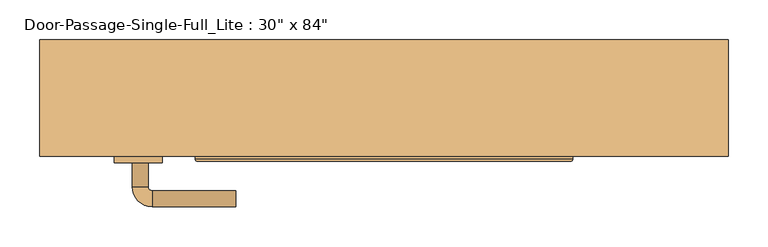
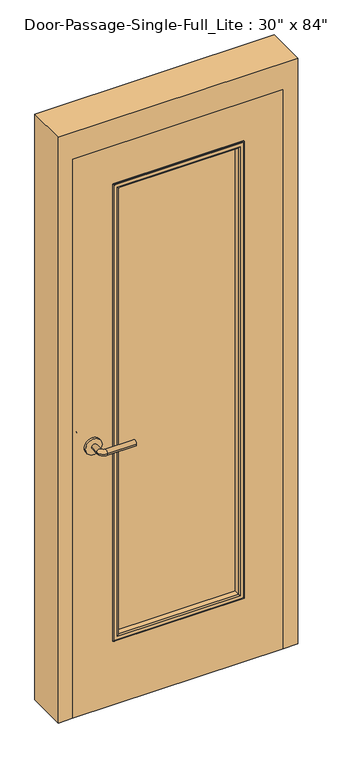
"""IFC4 building model written with IfcOpenShell, lengths in millimetres: door geometry."""

from ifc_helpers import new_model, si_unit, point, frame, frame_2d, origin, place, context, project, spatial, polyline, circle_curve, ellipse_curve, trimmed, segment, composite_curve, outline, extrude, faceted_brep, source, transform, mapped, element, save
from ifc_brep_helpers import plane_surface, cylinder_surface, revolved_surface, advanced_brep


def door_5d83ff76(model_context):
    return source(origin(), model_context, "Body", "SolidModel", [
        advanced_brep(
        [(-315.990625, -4.7, 1016.0), (-295.990625, -4.7, 1016.0), (-315.990625, 25.3, 1016.0), (-295.990625, 25.3, 1016.0), (-290.990625, 30.3, 1016.0), (-290.990625, 50.3, 1016.0), (-185.990625, 50.3, 1016.0), (-185.990625, 30.3, 1016.0)],
        [
            (0, 1, circle_curve(frame((-305.990625, -4.7, 1016.0), z_axis=(0.0, -1.0, 0.0), x_axis=(1.0, 0.0, 0.0)), 10.0)),
            (1, 0, circle_curve(frame((-305.990625, -4.7, 1016.0), z_axis=(0.0, -1.0, 0.0), x_axis=(1.0, 0.0, 0.0)), 10.0)),
            (0, 2),
            (2, 3, circle_curve(frame((-305.990625, 25.3, 1016.0), z_axis=(0.0, -1.0, 0.0), x_axis=(1.0, 0.0, 0.0)), 10.0)),
            (3, 1),
            (3, 2, circle_curve(frame((-305.990625, 25.3, 1016.0), z_axis=(0.0, -1.0, 0.0), x_axis=(1.0, 0.0, 0.0)), 10.0)),
            (4, 3, circle_curve(frame((-290.990625, 25.3, 1016.0), z_axis=(0.0, 0.0, 1.0), x_axis=(-1.0, 0.0, 0.0)), 5.0)),
            (2, 5, circle_curve(frame((-290.990625, 25.3, 1016.0), z_axis=(0.0, 0.0, -1.0), x_axis=(-1.0, 0.0, 0.0)), 25.0)),
            (5, 4, circle_curve(frame((-290.990625, 40.3, 1016.0), z_axis=(-1.0, 0.0, 0.0), x_axis=(0.0, -1.0, 0.0)), 10.0)),
            (4, 5, circle_curve(frame((-290.990625, 40.3, 1016.0), z_axis=(-1.0, 0.0, 0.0), x_axis=(0.0, -1.0, 0.0)), 10.0)),
            (6, 7, circle_curve(frame((-185.990625, 40.3, 1016.0), z_axis=(1.0, 0.0, 0.0), x_axis=(0.0, -1.0, 0.0)), 10.0)),
            (7, 6, circle_curve(frame((-185.990625, 40.3, 1016.0), z_axis=(1.0, 0.0, 0.0), x_axis=(0.0, -1.0, 0.0)), 10.0)),
            (5, 6),
            (7, 4),
        ],
        [
            plane_surface(frame((-305.990625, -4.7, 1016.0), z_axis=(0.0, -1.0, 0.0), x_axis=(0.0, 0.0, 1.0))),
            cylinder_surface(frame((-305.990625, -4.7, 1016.0), z_axis=(0.0, -1.0, 0.0), x_axis=(1.0, 0.0, 0.0)), 10.0),
            revolved_surface(trimmed(ellipse_curve(frame((-305.990625, 25.3, 1016.0), z_axis=(0.0, -1.0, 0.0), x_axis=(1.0, 0.0, 0.0)), 10.0, 10.0), [point((-315.990625, 25.3, 1016.0))], [point((-295.990625, 25.3, 1016.0))], True, "CARTESIAN"), (-290.990625, 25.3, 1016.0), (0.0, 0.0, -1.0)),
            revolved_surface(trimmed(ellipse_curve(frame((-305.990625, 25.3, 1016.0), z_axis=(0.0, -1.0, 0.0), x_axis=(1.0, 0.0, 0.0)), 10.0, 10.0), [point((-295.990625, 25.3, 1016.0))], [point((-315.990625, 25.3, 1016.0))], True, "CARTESIAN"), (-290.990625, 25.3, 1016.0), (0.0, 0.0, -1.0)),
            plane_surface(frame((-185.990625, 40.3, 1016.0), z_axis=(1.0, 0.0, 0.0), x_axis=(0.0, 0.0, 1.0))),
            cylinder_surface(frame((-290.990625, 40.3, 1016.0), z_axis=(-1.0, 0.0, 0.0), x_axis=(0.0, -1.0, 0.0)), 10.0),
        ],
        [
            (0, [[1, 2]]),
            (1, [[-1, 3, 4, 5]]),
            (1, [[-2, -5, 6, -3]]),
            (2, [[7, -4, 8, 9]]),
            (3, [[-8, -6, -7, 10]]),
            (4, [[11, 12]]),
            (5, [[-9, 13, -12, 14]]),
            (5, [[-10, -14, -11, -13]]),
        ],
    ),
        extrude(outline(composite_curve([segment(trimmed(circle_curve(frame_2d((1016.0, -308.490625)), 30.0), [point((1016.0, -338.490625))], [point((1016.0, -278.490625))], False, "CARTESIAN"), True, "CONTINUOUS"), segment(trimmed(circle_curve(frame_2d((1016.0, -308.490625)), 30.0), [point((1016.0, -278.490625))], [point((1016.0, -338.490625))], False, "CARTESIAN"), True, "CONTINUOUS")], self_intersect=False)), frame((0.0, -12.7, 0.0), z_axis=(0.0, 1.0, 0.0), x_axis=(0.0, 0.0, 1.0)), (0.0, 0.0, 1.0), 8.0),
        advanced_brep(
        [(-315.990625, -65.15, 1016.0), (-295.990625, -65.15, 1016.0), (-295.990625, -95.15, 1016.0), (-315.990625, -95.15, 1016.0), (-290.990625, -100.15, 1016.0), (-290.990625, -120.15, 1016.0), (-185.990625, -120.15, 1016.0), (-185.990625, -100.15, 1016.0)],
        [
            (0, 1, circle_curve(frame((-305.990625, -65.15, 1016.0), z_axis=(0.0, 1.0, 0.0), x_axis=(1.0, 0.0, 0.0)), 10.0)),
            (1, 0, circle_curve(frame((-305.990625, -65.15, 1016.0), z_axis=(0.0, 1.0, 0.0), x_axis=(1.0, 0.0, 0.0)), 10.0)),
            (1, 2),
            (2, 3, circle_curve(frame((-305.990625, -95.15, 1016.0), z_axis=(0.0, 1.0, 0.0), x_axis=(1.0, 0.0, 0.0)), 10.0)),
            (3, 0),
            (3, 2, circle_curve(frame((-305.990625, -95.15, 1016.0), z_axis=(0.0, 1.0, 0.0), x_axis=(1.0, 0.0, 0.0)), 10.0)),
            (4, 5, circle_curve(frame((-290.990625, -110.15, 1016.0), z_axis=(-1.0, 0.0, 0.0), x_axis=(0.0, 1.0, 0.0)), 10.0)),
            (5, 3, circle_curve(frame((-290.990625, -95.15, 1016.0), z_axis=(0.0, 0.0, -1.0), x_axis=(-1.0, 0.0, 0.0)), 25.0)),
            (2, 4, circle_curve(frame((-290.990625, -95.15, 1016.0), z_axis=(0.0, 0.0, 1.0), x_axis=(-1.0, 0.0, 0.0)), 5.0)),
            (5, 4, circle_curve(frame((-290.990625, -110.15, 1016.0), z_axis=(-1.0, 0.0, 0.0), x_axis=(0.0, 1.0, 0.0)), 10.0)),
            (6, 7, circle_curve(frame((-185.990625, -110.15, 1016.0), z_axis=(1.0, 0.0, 0.0), x_axis=(0.0, 1.0, 0.0)), 10.0)),
            (7, 6, circle_curve(frame((-185.990625, -110.15, 1016.0), z_axis=(1.0, 0.0, 0.0), x_axis=(0.0, 1.0, 0.0)), 10.0)),
            (4, 7),
            (6, 5),
        ],
        [
            plane_surface(frame((-305.990625, -65.15, 1016.0), z_axis=(0.0, 1.0, 0.0), x_axis=(0.0, 0.0, 1.0))),
            cylinder_surface(frame((-305.990625, -65.15, 1016.0), z_axis=(0.0, 1.0, 0.0), x_axis=(1.0, 0.0, 0.0)), 10.0),
            revolved_surface(trimmed(ellipse_curve(frame((-305.990625, -95.15, 1016.0), z_axis=(0.0, -1.0, 0.0), x_axis=(1.0, 0.0, 0.0)), 10.0, 10.0), [point((-315.990625, -95.15, 1016.0))], [point((-295.990625, -95.15, 1016.0))], True, "CARTESIAN"), (-290.990625, -95.15, 1016.0), (0.0, 0.0, -1.0)),
            revolved_surface(trimmed(ellipse_curve(frame((-305.990625, -95.15, 1016.0), z_axis=(0.0, -1.0, 0.0), x_axis=(1.0, 0.0, 0.0)), 10.0, 10.0), [point((-295.990625, -95.15, 1016.0))], [point((-315.990625, -95.15, 1016.0))], True, "CARTESIAN"), (-290.990625, -95.15, 1016.0), (0.0, 0.0, -1.0)),
            plane_surface(frame((-185.990625, -110.15, 1016.0), z_axis=(1.0, 0.0, 0.0), x_axis=(0.0, 0.0, 1.0))),
            cylinder_surface(frame((-290.990625, -110.15, 1016.0), z_axis=(-1.0, 0.0, 0.0), x_axis=(0.0, 1.0, 0.0)), 10.0),
        ],
        [
            (0, [[1, 2]]),
            (1, [[3, 4, 5, -2]]),
            (1, [[-5, 6, -3, -1]]),
            (2, [[7, 8, -4, 9]]),
            (3, [[10, -9, -6, -8]]),
            (4, [[11, 12]]),
            (5, [[13, -11, 14, -7]]),
            (5, [[-14, -12, -13, -10]]),
        ],
    ),
        extrude(outline(composite_curve([segment(trimmed(circle_curve(frame_2d((1016.0, -308.490625)), 30.0), [point((1016.0, -338.490625))], [point((1016.0, -278.490625))], False, "CARTESIAN"), True, "CONTINUOUS"), segment(trimmed(circle_curve(frame_2d((1016.0, -308.490625)), 30.0), [point((1016.0, -278.490625))], [point((1016.0, -338.490625))], False, "CARTESIAN"), True, "CONTINUOUS")], self_intersect=False)), frame((0.0, -65.15, 0.0), z_axis=(0.0, 1.0, 0.0), x_axis=(0.0, 0.0, 1.0)), (0.0, 0.0, 1.0), 8.0),
        extrude(outline(polyline([(228.6, -31.75), (228.6, -38.1), (-228.6, -38.1), (-228.6, -31.75), (228.6, -31.75)])), frame((0.0, 0.0, 254.0), z_axis=(0.0, 0.0, 1.0), x_axis=(1.0, 0.0, 0.0)), (0.0, 0.0, 1.0), 1727.2),
        faceted_brep([(381.0, -7.9375, 0.0), (365.125, -7.9375, 0.0), (365.125, 39.6875, 0.0), (381.0, 39.6875, 0.0), (381.0, 88.9, 0.0), (431.8, 88.9, 0.0), (431.8, -57.15, 0.0), (381.0, -57.15, 0.0), (381.0, -57.15, 2133.6), (381.0, -7.9375, 2133.6), (431.8, -57.15, 2235.2), (-431.8, -57.15, 2235.2), (-431.8, -57.15, 0.0), (-381.0, -57.15, 0.0), (-381.0, -57.15, 2133.6), (431.8, 88.9, 2235.2), (381.0, 88.9, 2133.6), (-381.0, 88.9, 2133.6), (-381.0, 88.9, 0.0), (-431.8, 88.9, 0.0), (-431.8, 88.9, 2235.2), (381.0, 39.6875, 2133.6), (365.125, 39.6875, 2117.725), (-365.125, 39.6875, 2117.725), (-365.125, 39.6875, 0.0), (-381.0, 39.6875, 0.0), (-381.0, 39.6875, 2133.6), (365.125, -7.9375, 2117.725), (-381.0, -7.9375, 2133.6), (-381.0, -7.9375, 0.0), (-365.125, -7.9375, 0.0), (-365.125, -7.9375, 2117.725)], [[[0, 1, 2, 3, 4, 5, 6, 7]], [[7, 8, 9, 0]], [[6, 10, 11, 12, 13, 14, 8, 7]], [[5, 15, 10, 6]], [[4, 16, 17, 18, 19, 20, 15, 5]], [[3, 21, 16, 4]], [[2, 22, 23, 24, 25, 26, 21, 3]], [[1, 27, 22, 2]], [[0, 9, 28, 29, 30, 31, 27, 1]], [[8, 14, 28, 9]], [[16, 21, 26, 17]], [[22, 27, 31, 23]], [[12, 19, 18, 25, 24, 30, 29, 13]], [[13, 29, 28, 14]], [[11, 20, 19, 12]], [[17, 26, 25, 18]], [[23, 31, 30, 24]], [[15, 20, 11, 10]]]),
        extrude(outline(polyline([(2133.6, -381.0), (0.0, -381.0), (0.0, 381.0), (2133.6, 381.0), (2133.6, -381.0)]), holes=[polyline([(1981.2, -228.6), (1981.2, 228.6), (254.0, 228.6), (254.0, -228.6), (1981.2, -228.6)])]), frame((0.0, -57.15, 0.0), z_axis=(0.0, 1.0, 0.0), x_axis=(0.0, 0.0, 1.0)), (0.0, 0.0, 1.0), 44.45),
        advanced_brep(
        [(-228.6, -38.1, 1981.2), (-228.6, -38.1, 254.0), (-228.6, -57.15, 254.0), (-228.6, -57.15, 1981.2), (-216.6, -58.15, 1969.2), (-216.6, -58.15, 266.0), (-216.6, -38.1, 266.0), (-216.6, -38.1, 1969.2), (-221.6, -63.15, 1974.2), (-221.6, -63.15, 261.0), (-236.6, -61.15, 1989.2), (-236.6, -61.15, 246.0), (-234.6, -63.15, 248.0), (-234.6, -63.15, 1987.2), (-236.6, -57.15, 1989.2), (-236.6, -57.15, 246.0), (228.6, -38.1, 254.0), (228.6, -57.15, 254.0), (216.6, -58.15, 266.0), (216.6, -38.1, 266.0), (221.6, -63.15, 261.0), (236.6, -61.15, 246.0), (234.6, -63.15, 248.0), (236.6, -57.15, 246.0), (228.6, -38.1, 1981.2), (228.6, -57.15, 1981.2), (216.6, -58.15, 1969.2), (216.6, -38.1, 1969.2), (221.6, -63.15, 1974.2), (236.6, -61.15, 1989.2), (234.6, -63.15, 1987.2), (236.6, -57.15, 1989.2)],
        [
            (0, 1),
            (1, 2),
            (2, 3),
            (3, 0),
            (4, 5),
            (5, 6),
            (6, 7),
            (7, 4),
            (8, 9),
            (9, 5, ellipse_curve(frame((-221.6, -58.15, 261.0), z_axis=(-0.7071067811865475, 0.0, 0.7071067811865475), x_axis=(0.7071067811865474, 0.0, 0.7071067811865476)), 7.0710678, 5.0)),
            (4, 8, ellipse_curve(frame((-221.6, -58.15, 1974.2), z_axis=(-0.7071067811865475, 0.0, -0.7071067811865475), x_axis=(-0.7071067811865474, 0.0, 0.7071067811865476)), 7.0710678, 5.0)),
            (10, 11),
            (11, 12, ellipse_curve(frame((-234.6, -61.15, 248.0), z_axis=(-0.7071067811865475, 0.0, 0.7071067811865475), x_axis=(0.7071067811865474, 0.0, 0.7071067811865476)), 2.8284271, 2.0)),
            (12, 13),
            (13, 10, ellipse_curve(frame((-234.6, -61.15, 1987.2), z_axis=(-0.7071067811865475, 0.0, -0.7071067811865475), x_axis=(-0.7071067811865474, 0.0, 0.7071067811865476)), 2.8284271, 2.0)),
            (14, 15),
            (15, 11),
            (10, 14),
            (1, 16),
            (16, 17),
            (17, 2),
            (5, 18),
            (18, 19),
            (19, 6),
            (9, 20),
            (20, 18, ellipse_curve(frame((221.6, -58.15, 261.0), z_axis=(-0.7071067811865475, 0.0, -0.7071067811865475), x_axis=(-0.7071067811865476, 0.0, 0.7071067811865474)), 7.0710678, 5.0)),
            (11, 21),
            (21, 22, ellipse_curve(frame((234.6, -61.15, 248.0), z_axis=(-0.7071067811865475, 0.0, -0.7071067811865475), x_axis=(-0.7071067811865476, 0.0, 0.7071067811865474)), 2.8284271, 2.0)),
            (22, 12),
            (15, 23),
            (23, 21),
            (16, 24),
            (24, 25),
            (25, 17),
            (18, 26),
            (26, 27),
            (27, 19),
            (20, 28),
            (28, 26, ellipse_curve(frame((221.6, -58.15, 1974.2), z_axis=(0.7071067811865475, 0.0, -0.7071067811865475), x_axis=(-0.7071067811865474, 0.0, -0.7071067811865476)), 7.0710678, 5.0)),
            (21, 29),
            (29, 30, ellipse_curve(frame((234.6, -61.15, 1987.2), z_axis=(0.7071067811865475, 0.0, -0.7071067811865475), x_axis=(-0.7071067811865474, 0.0, -0.7071067811865476)), 2.8284271, 2.0)),
            (30, 22),
            (23, 31),
            (31, 29),
            (14, 31),
            (25, 3),
            (24, 0),
            (27, 7),
            (26, 4),
            (28, 8),
            (30, 13),
            (29, 10),
        ],
        [
            plane_surface(frame((-228.6, -57.15, 1981.2), z_axis=(-1.0, 0.0, 0.0), x_axis=(0.0, 0.0, -1.0))),
            plane_surface(frame((-216.6, -38.1, 1969.2), z_axis=(1.0, 0.0, 0.0), x_axis=(0.0, 0.0, -1.0))),
            cylinder_surface(frame((-221.6, -58.15, 1981.2), z_axis=(0.0, 0.0, 1.0), x_axis=(-1.0, 0.0, 0.0)), 5.0),
            cylinder_surface(frame((-234.6, -61.15, 1981.2), z_axis=(0.0, 0.0, 1.0), x_axis=(-1.0, 0.0, 0.0)), 2.0),
            plane_surface(frame((-236.6, -61.15, 1989.2), z_axis=(-1.0, 0.0, 0.0), x_axis=(0.0, 0.0, -1.0))),
            plane_surface(frame((-228.6, -57.15, 254.0), z_axis=(0.0, 0.0, -1.0), x_axis=(1.0, 0.0, 0.0))),
            plane_surface(frame((-216.6, -38.1, 266.0), z_axis=(0.0, 0.0, 1.0), x_axis=(1.0, 0.0, 0.0))),
            cylinder_surface(frame((-228.6, -58.15, 261.0), z_axis=(-1.0, 0.0, 0.0), x_axis=(0.0, 0.0, -1.0)), 5.0),
            cylinder_surface(frame((-228.6, -61.15, 248.0), z_axis=(-1.0, 0.0, 0.0), x_axis=(0.0, 0.0, -1.0)), 2.0),
            plane_surface(frame((-236.6, -61.15, 246.0), z_axis=(0.0, 0.0, -1.0), x_axis=(1.0, 0.0, 0.0))),
            plane_surface(frame((228.6, -57.15, 254.0), z_axis=(1.0, 0.0, 0.0), x_axis=(0.0, 0.0, 1.0))),
            plane_surface(frame((216.6, -38.1, 266.0), z_axis=(-1.0, 0.0, 0.0), x_axis=(0.0, 0.0, 1.0))),
            cylinder_surface(frame((221.6, -58.15, 254.0), z_axis=(0.0, 0.0, -1.0), x_axis=(1.0, 0.0, 0.0)), 5.0),
            cylinder_surface(frame((234.6, -61.15, 254.0), z_axis=(0.0, 0.0, -1.0), x_axis=(1.0, 0.0, 0.0)), 2.0),
            plane_surface(frame((236.6, -61.15, 246.0), z_axis=(1.0, 0.0, 0.0), x_axis=(0.0, 0.0, 1.0))),
            plane_surface(frame((236.6, -57.15, 1989.2), z_axis=(0.0, 1.0, 0.0), x_axis=(-1.0, 0.0, 0.0))),
            plane_surface(frame((228.6, -57.15, 1981.2), z_axis=(0.0, 0.0, 1.0), x_axis=(-1.0, 0.0, 0.0))),
            plane_surface(frame((228.6, -38.1, 1981.2), z_axis=(0.0, 1.0, 0.0), x_axis=(-1.0, 0.0, 0.0))),
            plane_surface(frame((216.6, -38.1, 1969.2), z_axis=(0.0, 0.0, -1.0), x_axis=(-1.0, 0.0, 0.0))),
            cylinder_surface(frame((228.6, -58.15, 1974.2), z_axis=(1.0, 0.0, 0.0), x_axis=(0.0, 0.0, 1.0)), 5.0),
            plane_surface(frame((221.6, -63.15, 1974.2), z_axis=(0.0, -1.0, 0.0), x_axis=(-1.0, 0.0, 0.0))),
            cylinder_surface(frame((228.6, -61.15, 1987.2), z_axis=(1.0, 0.0, 0.0), x_axis=(0.0, 0.0, 1.0)), 2.0),
            plane_surface(frame((236.6, -61.15, 1989.2), z_axis=(0.0, 0.0, 1.0), x_axis=(-1.0, 0.0, 0.0))),
        ],
        [
            (0, [[1, 2, 3, 4]]),
            (1, [[5, 6, 7, 8]]),
            (2, [[9, 10, -5, 11]]),
            (3, [[12, 13, 14, 15]]),
            (4, [[16, 17, -12, 18]]),
            (5, [[19, 20, 21, -2]]),
            (6, [[22, 23, 24, -6]]),
            (7, [[25, 26, -22, -10]]),
            (8, [[27, 28, 29, -13]]),
            (9, [[30, 31, -27, -17]]),
            (10, [[32, 33, 34, -20]]),
            (11, [[35, 36, 37, -23]]),
            (12, [[38, 39, -35, -26]]),
            (13, [[40, 41, 42, -28]]),
            (14, [[43, 44, -40, -31]]),
            (15, [[-16, 45, -43, -30], [-3, -21, -34, 46]]),
            (16, [[47, -4, -46, -33]]),
            (17, [[-1, -47, -32, -19], [-7, -24, -37, 48]]),
            (18, [[49, -8, -48, -36]]),
            (19, [[50, -11, -49, -39]]),
            (20, [[-14, -29, -42, 51], [-9, -50, -38, -25]]),
            (21, [[52, -15, -51, -41]]),
            (22, [[-45, -18, -52, -44]]),
        ],
    ),
        advanced_brep(
        [(-228.6, -31.75, 254.0), (-228.6, -31.75, 1981.2), (-228.6, -12.7, 1981.2), (-228.6, -12.7, 254.0), (-216.6, -11.7, 266.0), (-216.6, -11.7, 1969.2), (-216.6, -31.75, 1969.2), (-216.6, -31.75, 266.0), (-221.6, -6.7, 261.0), (-221.6, -6.7, 1974.2), (-236.6, -8.7, 246.0), (-236.6, -8.7, 1989.2), (-234.6, -6.7, 1987.2), (-234.6, -6.7, 248.0), (-236.6, -12.7, 246.0), (-236.6, -12.7, 1989.2), (228.6, -31.75, 1981.2), (228.6, -12.7, 1981.2), (216.6, -11.7, 1969.2), (216.6, -31.75, 1969.2), (221.6, -6.7, 1974.2), (236.6, -8.7, 1989.2), (234.6, -6.7, 1987.2), (236.6, -12.7, 1989.2), (228.6, -31.75, 254.0), (228.6, -12.7, 254.0), (216.6, -11.7, 266.0), (216.6, -31.75, 266.0), (221.6, -6.7, 261.0), (236.6, -8.7, 246.0), (234.6, -6.7, 248.0), (236.6, -12.7, 246.0)],
        [
            (0, 1),
            (1, 2),
            (2, 3),
            (3, 0),
            (4, 5),
            (5, 6),
            (6, 7),
            (7, 4),
            (8, 9),
            (9, 5, ellipse_curve(frame((-221.6, -11.7, 1974.2), z_axis=(-0.7071067811865475, 0.0, -0.7071067811865475), x_axis=(0.7071067811865474, 0.0, -0.7071067811865476)), 7.0710678, 5.0)),
            (4, 8, ellipse_curve(frame((-221.6, -11.7, 261.0), z_axis=(-0.7071067811865475, 0.0, 0.7071067811865475), x_axis=(-0.7071067811865474, 0.0, -0.7071067811865476)), 7.0710678, 5.0)),
            (10, 11),
            (11, 12, ellipse_curve(frame((-234.6, -8.7, 1987.2), z_axis=(-0.7071067811865475, 0.0, -0.7071067811865475), x_axis=(0.7071067811865474, 0.0, -0.7071067811865476)), 2.8284271, 2.0)),
            (12, 13),
            (13, 10, ellipse_curve(frame((-234.6, -8.7, 248.0), z_axis=(-0.7071067811865475, 0.0, 0.7071067811865475), x_axis=(-0.7071067811865474, 0.0, -0.7071067811865476)), 2.8284271, 2.0)),
            (14, 15),
            (15, 11),
            (10, 14),
            (1, 16),
            (16, 17),
            (17, 2),
            (5, 18),
            (18, 19),
            (19, 6),
            (9, 20),
            (20, 18, ellipse_curve(frame((221.6, -11.7, 1974.2), z_axis=(-0.7071067811865475, 0.0, 0.7071067811865475), x_axis=(-0.7071067811865476, 0.0, -0.7071067811865474)), 7.0710678, 5.0)),
            (11, 21),
            (21, 22, ellipse_curve(frame((234.6, -8.7, 1987.2), z_axis=(-0.7071067811865475, 0.0, 0.7071067811865475), x_axis=(-0.7071067811865476, 0.0, -0.7071067811865474)), 2.8284271, 2.0)),
            (22, 12),
            (15, 23),
            (23, 21),
            (16, 24),
            (24, 25),
            (25, 17),
            (18, 26),
            (26, 27),
            (27, 19),
            (20, 28),
            (28, 26, ellipse_curve(frame((221.6, -11.7, 261.0), z_axis=(0.7071067811865475, 0.0, 0.7071067811865475), x_axis=(-0.7071067811865474, 0.0, 0.7071067811865476)), 7.0710678, 5.0)),
            (21, 29),
            (29, 30, ellipse_curve(frame((234.6, -8.7, 248.0), z_axis=(0.7071067811865475, 0.0, 0.7071067811865475), x_axis=(-0.7071067811865474, 0.0, 0.7071067811865476)), 2.8284271, 2.0)),
            (30, 22),
            (23, 31),
            (31, 29),
            (14, 31),
            (25, 3),
            (24, 0),
            (27, 7),
            (26, 4),
            (28, 8),
            (30, 13),
            (29, 10),
        ],
        [
            plane_surface(frame((-228.6, -12.7, 254.0), z_axis=(-1.0, 0.0, 0.0), x_axis=(0.0, 0.0, 1.0))),
            plane_surface(frame((-216.6, -31.75, 266.0), z_axis=(1.0, 0.0, 0.0), x_axis=(0.0, 0.0, 1.0))),
            cylinder_surface(frame((-221.6, -11.7, 254.0), z_axis=(0.0, 0.0, -1.0), x_axis=(-1.0, 0.0, 0.0)), 5.0),
            cylinder_surface(frame((-234.6, -8.7, 254.0), z_axis=(0.0, 0.0, -1.0), x_axis=(-1.0, 0.0, 0.0)), 2.0),
            plane_surface(frame((-236.6, -8.7, 246.0), z_axis=(-1.0, 0.0, 0.0), x_axis=(0.0, 0.0, 1.0))),
            plane_surface(frame((-228.6, -12.7, 1981.2), z_axis=(0.0, 0.0, 1.0), x_axis=(1.0, 0.0, 0.0))),
            plane_surface(frame((-216.6, -31.75, 1969.2), z_axis=(0.0, 0.0, -1.0), x_axis=(1.0, 0.0, 0.0))),
            cylinder_surface(frame((-228.6, -11.7, 1974.2), z_axis=(-1.0, 0.0, 0.0), x_axis=(0.0, 0.0, 1.0)), 5.0),
            cylinder_surface(frame((-228.6, -8.7, 1987.2), z_axis=(-1.0, 0.0, 0.0), x_axis=(0.0, 0.0, 1.0)), 2.0),
            plane_surface(frame((-236.6, -8.7, 1989.2), z_axis=(0.0, 0.0, 1.0), x_axis=(1.0, 0.0, 0.0))),
            plane_surface(frame((228.6, -12.7, 1981.2), z_axis=(1.0, 0.0, 0.0), x_axis=(0.0, 0.0, -1.0))),
            plane_surface(frame((216.6, -31.75, 1969.2), z_axis=(-1.0, 0.0, 0.0), x_axis=(0.0, 0.0, -1.0))),
            cylinder_surface(frame((221.6, -11.7, 1981.2), z_axis=(0.0, 0.0, 1.0), x_axis=(1.0, 0.0, 0.0)), 5.0),
            cylinder_surface(frame((234.6, -8.7, 1981.2), z_axis=(0.0, 0.0, 1.0), x_axis=(1.0, 0.0, 0.0)), 2.0),
            plane_surface(frame((236.6, -8.7, 1989.2), z_axis=(1.0, 0.0, 0.0), x_axis=(0.0, 0.0, -1.0))),
            plane_surface(frame((236.6, -12.7, 246.0), z_axis=(0.0, -1.0, 0.0), x_axis=(-1.0, 0.0, 0.0))),
            plane_surface(frame((228.6, -12.7, 254.0), z_axis=(0.0, 0.0, -1.0), x_axis=(-1.0, 0.0, 0.0))),
            plane_surface(frame((228.6, -31.75, 254.0), z_axis=(0.0, -1.0, 0.0), x_axis=(-1.0, 0.0, 0.0))),
            plane_surface(frame((216.6, -31.75, 266.0), z_axis=(0.0, 0.0, 1.0), x_axis=(-1.0, 0.0, 0.0))),
            cylinder_surface(frame((228.6, -11.7, 261.0), z_axis=(1.0, 0.0, 0.0), x_axis=(0.0, 0.0, -1.0)), 5.0),
            plane_surface(frame((221.6, -6.7, 261.0), z_axis=(0.0, 1.0, 0.0), x_axis=(-1.0, 0.0, 0.0))),
            cylinder_surface(frame((228.6, -8.7, 248.0), z_axis=(1.0, 0.0, 0.0), x_axis=(0.0, 0.0, -1.0)), 2.0),
            plane_surface(frame((236.6, -8.7, 246.0), z_axis=(0.0, 0.0, -1.0), x_axis=(-1.0, 0.0, 0.0))),
        ],
        [
            (0, [[1, 2, 3, 4]]),
            (1, [[5, 6, 7, 8]]),
            (2, [[9, 10, -5, 11]]),
            (3, [[12, 13, 14, 15]]),
            (4, [[16, 17, -12, 18]]),
            (5, [[19, 20, 21, -2]]),
            (6, [[22, 23, 24, -6]]),
            (7, [[25, 26, -22, -10]]),
            (8, [[27, 28, 29, -13]]),
            (9, [[30, 31, -27, -17]]),
            (10, [[32, 33, 34, -20]]),
            (11, [[35, 36, 37, -23]]),
            (12, [[38, 39, -35, -26]]),
            (13, [[40, 41, 42, -28]]),
            (14, [[43, 44, -40, -31]]),
            (15, [[-16, 45, -43, -30], [-3, -21, -34, 46]]),
            (16, [[47, -4, -46, -33]]),
            (17, [[-1, -47, -32, -19], [-7, -24, -37, 48]]),
            (18, [[49, -8, -48, -36]]),
            (19, [[50, -11, -49, -39]]),
            (20, [[-14, -29, -42, 51], [-9, -50, -38, -25]]),
            (21, [[52, -15, -51, -41]]),
            (22, [[-45, -18, -52, -44]]),
        ],
    ),
    ])


if __name__ == "__main__":
    model = new_model("IFC4")
    model_context = context("Model", 3, world=origin())
    ifc_project = project(units=[si_unit("LENGTHUNIT", "METRE", prefix="MILLI")], contexts=[model_context])
    site = spatial("IfcSite", under=ifc_project)
    building = spatial("IfcBuilding", under=site)
    placement = place(None, origin())
    door_shape = door_5d83ff76(model_context)
    element("IfcDoor", 1, ObjectType="Door-Passage-Single-Full_Lite : 30\" x 84\"", at=placement, inside=building, context=model_context, shape_type="MappedRepresentation", body=[
        mapped(door_shape, transform((0.0, 0.0, 0.0), x_axis=(1.0, 0.0, 0.0), y_axis=(0.0, 1.0, 0.0), z_axis=(0.0, 0.0, 1.0))),
    ])
    save(model, "model.ifc")

# Revit data of these elements
# Type "Door-Passage-Single-Full_Lite : 30\" x 84\""
#   Type Mark = "9"
#   Assembly Code = "B2030100"
#   Analytic Construction = "Wooden"
#   Thickness = 0' - 1 3/4"
#   Thermal Resistance (R) = 2.5876 (h·ft²·°F)/BTU
#   Swing Angle [instance default] = 90.00°
#   Strike Height = 3' - 4"
#   Rough Width [instance default] = 2' - 10"
#   Rough Height [instance default] = 7' - 4"
#   MF Opening Height [instance default] = 0' - 4"
#   MF Opening Width [instance default] = 0' - 4"
#   Inset Calculate [instance default] = 0' - 4"
#   Masonry Inset [instance default] = 0' - 1"
#   Height = 7' - 0"
#   Width = 2' - 6"
#   Heat Transfer Coefficient (U) = 0.3865 BTU/(h·ft²·°F)
#   Masonry Frame Depth = 0' - 5 3/4"
#   Masonry Frame [instance default] = yes
#   Function = 1
#   Dry Wall Frame [instance default] = no
#   Panel Material = Wood - Birch
#   Glazing = Glass
#   Glass Stop Material = Metal - Paint Finish - Grey
#   Frame Material = Metal - Paint Finish - Grey
#   Door Handle Material = Aluminum
#   Visual Light Transmittance = 0
#   Solar Heat Gain Coefficient = 0
#   Wall Closure = (empty or 0)
# Element 1 (IfcDoor, "Door-Passage-Single-Full_Lite : 30\" x 84\"")
#   Materials on its faces: "Metal - Paint Finish - Grey", "Aluminum", "Wood - Birch", "Glass"
# Materials
#   "Wood - Birch": class "Wood", colour RGB 166 116 52, transparency 0, Cost = 0
#   "Glass": class "Glass", colour RGB 0 128 192, transparency 0.75, Description = "Soda Lime Glass", Cost = 0
#   "Metal - Paint Finish - Grey": class "Paint", colour RGB 104 104 104, transparency 0, Cost = 0
#   "Aluminum": class "Metal", colour RGB 247 247 247, transparency 0, Description = "Aluminum 6061", Cost = 0
